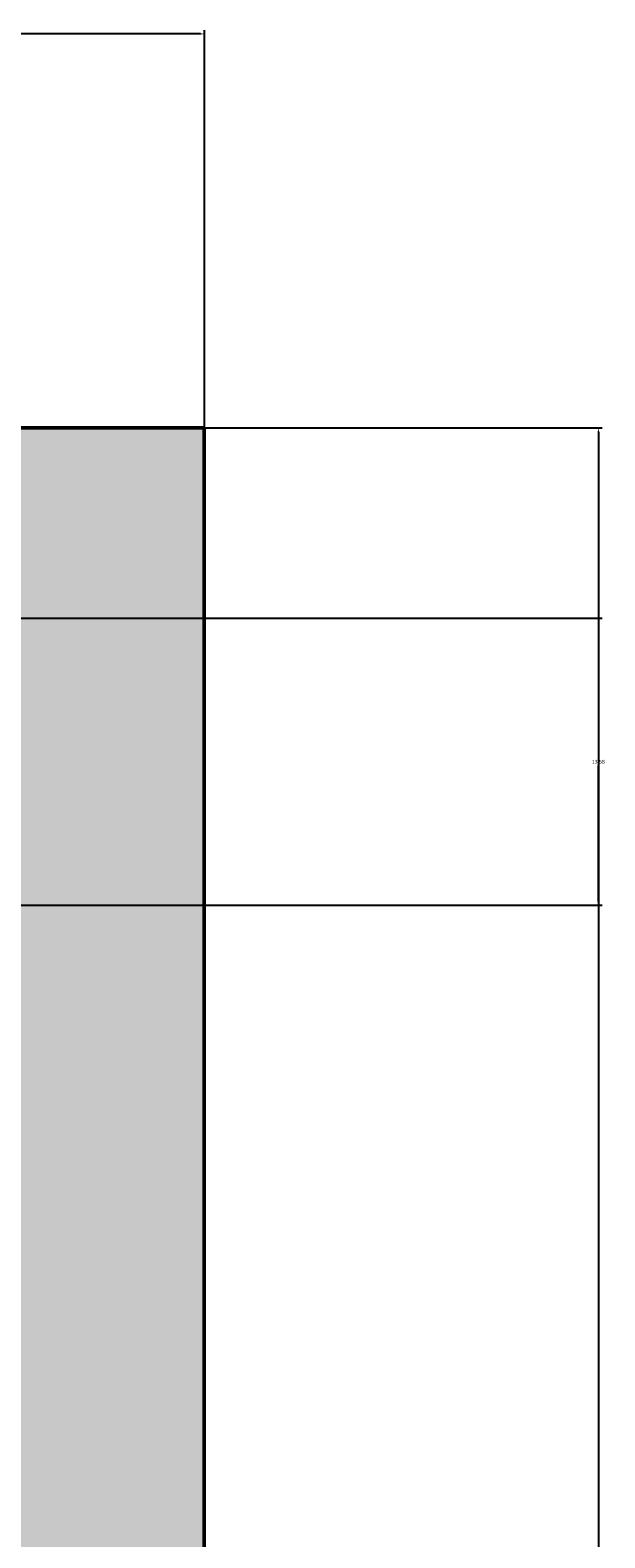
# Model space of a CAD drawing. Units: inches. Extents: x 2231 to 2461, y 2045 to 2455.
# Tile 95 of 95: x 2434 to 2461, y 2383 to 2455. Entities that reach past the tile are written whole.
import ezdxf

# ---------------------------------------------------------------- set-up
doc = ezdxf.new("R2010")
doc.units = ezdxf.units.IN
doc.layers.add('A-ANNO-DIMS', color=2, linetype='Continuous', lineweight=18)
doc.layers.add('A-WALL', color=7, linetype='Continuous', lineweight=50)
doc.layers.add('A-WALL-PATT', color=18, linetype='Continuous', lineweight=13, true_color=0x000000)
doc.styles.get("Standard").update_dxf_attribs({"font": 'arial.ttf'})
doc.dimstyles.get("Standard").update_dxf_attribs({"dimtxt": 0.18, "dimasz": 0.18, "dimexe": 0.18, "dimexo": 0.0625, "dimgap": 0.09, "dimtad": 0, "dimtih": 1, "dimtoh": 1, "dimdec": 4, "dimzin": 0, "dimdsep": 46, "dimtxsty": 'Standard', "dimcen": 0.09, "dimadec": 0, "dimazin": 0, "dimtfac": 1, "dimtdec": 4, "dimtofl": 0, "dimtmove": 0, "dimatfit": 3, "dimfxl": 1, "dimtolj": 1, "dimtzin": 0, "dimarcsym": 0})

# ---------------------------------------------------------------- blocks, each defined once
blk = doc.blocks.new('*D34')
at = {"layer": 'A-ANNO-DIMS', "color": 0, "lineweight": -2, "transparency": 16777216}
for p, q in [((2441.856, 2435.833), (2460.606, 2435.833)), ((2460.426, 2435.653), (2460.426, 2250.015)), ((2460.426, 2064.013), (2460.426, 2249.651)), ((2441.856, 2063.833), (2460.606, 2063.833))]:
    blk.add_line(p, q, dxfattribs=at)
at = {"layer": 'A-ANNO-DIMS', "color": 0, "transparency": 16777216}
for points in [[(2460.396, 2435.653), (2460.456, 2435.653), (2460.426, 2435.833)], [(2460.396, 2064.013), (2460.456, 2064.013), (2460.426, 2063.833)]]:
    blk.add_solid(points, dxfattribs=at)
at = {"layer": 'Defpoints', "color": 0, "transparency": 16777216}
for p in [(2441.794, 2435.833), (2460.426, 2435.833), (2441.794, 2063.833)]:
    blk.add_point(p, dxfattribs=at)
at = {"layer": 'A-ANNO-DIMS', "color": 0, "transparency": 16777216, "insert": (2460.426, 2249.833), "char_height": 0.18, "attachment_point": 5}
blk.add_mtext('\\A1;372', dxfattribs=at)
blk = doc.blocks.new('*D38')
at = {"layer": 'A-ANNO-DIMS', "color": 0, "lineweight": -2, "transparency": 16777216}
for p, q in [((2432.856, 2426.833), (2460.606, 2426.833)), ((2460.426, 2426.653), (2460.426, 2381.015)), ((2460.426, 2335.013), (2460.426, 2380.651)), ((2432.856, 2334.833), (2460.606, 2334.833))]:
    blk.add_line(p, q, dxfattribs=at)
at = {"layer": 'A-ANNO-DIMS', "color": 0, "transparency": 16777216}
for points in [[(2460.396, 2426.653), (2460.456, 2426.653), (2460.426, 2426.833)], [(2460.396, 2335.013), (2460.456, 2335.013), (2460.426, 2334.833)]]:
    blk.add_solid(points, dxfattribs=at)
at = {"layer": 'Defpoints', "color": 0, "transparency": 16777216}
for p in [(2432.794, 2426.833), (2460.426, 2426.833), (2432.794, 2334.833)]:
    blk.add_point(p, dxfattribs=at)
at = {"layer": 'A-ANNO-DIMS', "color": 0, "transparency": 16777216, "insert": (2460.426, 2380.833), "char_height": 0.18, "attachment_point": 5}
blk.add_mtext('\\A1;92', dxfattribs=at)
blk = doc.blocks.new('*D56')
at = {"layer": 'A-ANNO-DIMS', "color": 0, "lineweight": -2, "transparency": 16777216}
for p, q in [((2415.934, 2435.895), (2415.934, 2454.645)), ((2416.114, 2454.465), (2428.468, 2454.465)), ((2441.614, 2454.465), (2429.259, 2454.465)), ((2441.794, 2435.895), (2441.794, 2454.645))]:
    blk.add_line(p, q, dxfattribs=at)
at = {"layer": 'A-ANNO-DIMS', "color": 0, "transparency": 16777216}
for points in [[(2416.114, 2454.495), (2416.114, 2454.435), (2415.934, 2454.465)], [(2441.614, 2454.495), (2441.614, 2454.435), (2441.794, 2454.465)]]:
    blk.add_solid(points, dxfattribs=at)
at = {"layer": 'Defpoints', "color": 0, "transparency": 16777216}
for p in [(2441.794, 2454.465), (2415.934, 2435.833), (2441.794, 2435.833)]:
    blk.add_point(p, dxfattribs=at)
at = {"layer": 'A-ANNO-DIMS', "color": 0, "transparency": 16777216, "insert": (2428.864, 2454.465), "char_height": 0.18, "attachment_point": 5}
blk.add_mtext('\\A1;25.86', dxfattribs=at)
blk = doc.blocks.new('*D68')
at = {"layer": 'A-ANNO-DIMS', "color": 0, "lineweight": -2, "transparency": 16777216}
for p, q in [((2285.882, 2426.833), (2460.606, 2426.833)), ((2460.426, 2426.653), (2460.426, 2420.225)), ((2460.426, 2413.433), (2460.426, 2419.861)), ((2278.251, 2413.253), (2460.606, 2413.253))]:
    blk.add_line(p, q, dxfattribs=at)
at = {"layer": 'A-ANNO-DIMS', "color": 0, "transparency": 16777216}
for points in [[(2460.396, 2426.653), (2460.456, 2426.653), (2460.426, 2426.833)], [(2460.396, 2413.433), (2460.456, 2413.433), (2460.426, 2413.253)]]:
    blk.add_solid(points, dxfattribs=at)
at = {"layer": 'Defpoints', "color": 0, "transparency": 16777216}
for p in [(2285.82, 2426.833), (2460.426, 2426.833), (2278.188, 2413.253)]:
    blk.add_point(p, dxfattribs=at)
at = {"layer": 'A-ANNO-DIMS', "color": 0, "transparency": 16777216, "insert": (2460.426, 2420.043), "char_height": 0.18, "attachment_point": 5}
blk.add_mtext('\\A1;13.58', dxfattribs=at)

msp = doc.modelspace()

# ---------------------------------------------------------------- hatches: boundary and pattern name
at = {"layer": 'A-WALL-PATT'}
h = msp.add_hatch(color=256, dxfattribs=at)
h.dxf.hatch_style = 1
h.paths.add_polyline_path([(2441.7935, 2269.1535), (2432.7935, 2269.1535), (2432.7935, 2186.8328), (2396.7935, 2186.8328), (2396.7935, 2286.8328), (2394.7935, 2286.8328), (2394.7935, 2186.8328), (2334.7935, 2186.8328), (2334.7935, 2182.8328), (2432.7935, 2182.8328), (2432.7935, 2072.8328), (2416.6639, 2072.8328), (2416.6639, 2063.8328), (2441.7935, 2063.8328)])
h.paths.add_polyline_path([(2368.6639, 2072.8328), (2367.04, 2072.8328), (2330.7942, 2072.8328), (2330.7397, 2063.8328), (2368.6639, 2063.8328)])
h.paths.add_polyline_path([(2300.7392, 2068.3328), (2300.7392, 2072.8328), (2298.7935, 2072.8328), (2294.7935, 2072.8328), (2258.7935, 2072.8328), (2258.7935, 2120.8328), (2294.7935, 2120.8328), (2298.7935, 2120.8328), (2298.7935, 2128.8328), (2294.7935, 2128.8328), (2294.7935, 2124.8328), (2258.7935, 2124.8328), (2258.7935, 2182.8328), (2294.7935, 2182.8328), (2294.7935, 2174.8328), (2298.7935, 2174.8328), (2298.7935, 2182.8328), (2304.7935, 2182.8328), (2304.7935, 2186.8328), (2258.7935, 2186.8328), (2258.7935, 2221.999), (2249.7935, 2221.999), (2249.7935, 2063.8328), (2300.7392, 2063.8328)])
h.paths.add_polyline_path([(2391.9338, 2435.8328), (2333.82, 2435.8328), (2333.82, 2426.8328), (2368.7935, 2426.8328), (2368.7935, 2374.9508), (2368.7935, 2370.8328), (2372.3935, 2370.8328), (2372.7935, 2370.8328), (2372.7935, 2426.8328), (2391.9338, 2426.8328)])
h.paths.add_polyline_path([(2441.7935, 2435.8328), (2415.9338, 2435.8328), (2415.9338, 2426.8328), (2432.7935, 2426.8328), (2432.7935, 2334.8328), (2372.7935, 2334.8328), (2372.7935, 2346.8328), (2368.7935, 2346.8328), (2368.7935, 2306.8328), (2360.7935, 2306.8328), (2360.7935, 2302.8328), (2368.7935, 2302.8328), (2372.7935, 2302.8328), (2372.7935, 2330.8328), (2432.7935, 2330.8328), (2432.7935, 2317.1535), (2441.7935, 2317.1535)])
h.paths.add_polyline_path([(2285.82, 2435.8328), (2249.7935, 2435.8328), (2249.7935, 2269.999), (2258.7935, 2269.999), (2258.7935, 2302.8328), (2318.8168, 2302.8328), (2330.7935, 2302.8328), (2330.7935, 2306.8328), (2258.7935, 2306.8328), (2258.7935, 2426.8328), (2285.82, 2426.8328)])

# ---------------------------------------------------------------- linework, layer by layer
at = {"layer": 'A-WALL'}
msp.add_lwpolyline([(2300.7392, 2063.8328), (2249.7935, 2063.8328), (2249.7935, 2435.8328), (2441.7935, 2435.8328), (2441.7935, 2063.8328), (2330.7397, 2063.8328)], dxfattribs=at)

# ---------------------------------------------------------------- dimensions: what is measured, and where the dimension line sits
at = {"layer": 'A-ANNO-DIMS'}
dim = msp.add_linear_dim(base=(2441.7935, 2454.4653), p1=(2415.9338, 2435.8328), p2=(2441.7935, 2435.8328), dimstyle='Standard', override={"dimdec": 2, "dimlfac": 1, "dimrnd": 0, "dimzin": 0, "dimdsep": 46, "dimlunit": 2}, dxfattribs=at)
dim.commit()
dim.dimension.update_dxf_attribs({"geometry": '*D56', "text_midpoint": (2428.8637, 2454.4653)})
for base, p1, p2, override, picture, middle in [((2460.426, 2435.8328), (2441.7935, 2063.8328), (2441.7935, 2435.8328), {"dimdec": 0, "dimlfac": 1, "dimrnd": 0, "dimzin": 0, "dimdsep": 46, "dimlunit": 2}, '*D34', (2460.426, 2249.8328)), ((2460.426, 2426.8328), (2278.1881, 2413.2534), (2285.82, 2426.8328), {"dimdec": 2, "dimlfac": 1, "dimrnd": 0, "dimzin": 0, "dimdsep": 46, "dimlunit": 2}, '*D68', (2460.426, 2420.0431)), ((2460.426, 2426.8328), (2432.7935, 2334.8328), (2432.7935, 2426.8328), {"dimdec": 0, "dimlfac": 1, "dimrnd": 0, "dimzin": 0, "dimdsep": 46, "dimlunit": 2}, '*D38', (2460.426, 2380.8328))]:
    dim = msp.add_linear_dim(base=base, p1=p1, p2=p2, angle=90, dimstyle='Standard', override=override, dxfattribs=at)
    dim.commit()
    dim.dimension.update_dxf_attribs({"geometry": picture, "text_midpoint": middle})

doc.saveas('drawing.dxf')
